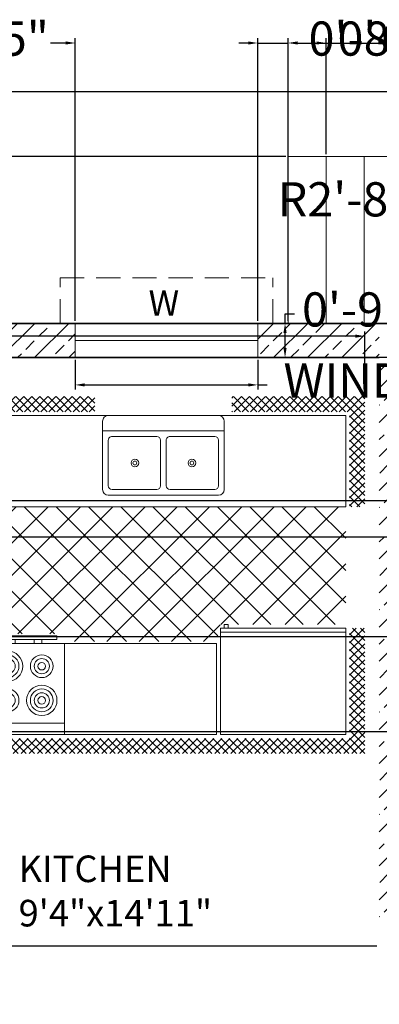
# Model space of a CAD drawing. Units: inches. Extents: x 9689 to 10369, y 10965 to 11626.
# Tile 6 of 11: x 9828 to 9923, y 11359 to 11619. Entities that reach past the tile are written whole.
import ezdxf

# ---------------------------------------------------------------- set-up
doc = ezdxf.new("R2010")
doc.units = ezdxf.units.IN
doc.linetypes.add('DASHED2', pattern=[9.525, 6.35, -3.175])
for name, color, linetype, lineweight in [('A-ANNO-DIMS', 2, 'Continuous', 18), ('A-ANNO-TEXT', 7, 'Continuous', 18), ('A-AREA-IDEN', 7, 'Continuous', 18), ('A-FLOR-FIXT', 8, 'Continuous', 18), ('A-FLOR-STRS', 7, 'Continuous', 18), ('A-GLAZ', 4, 'Continuous', 18), ('A-GLAZ-OVHD', 4, 'DASHED2', 13), ('A-WALL', 7, 'Continuous', 35), ('A-WALL-PATT', 252, 'Continuous', 13)]:
    doc.layers.add(name, color=color, linetype=linetype, lineweight=lineweight)
doc.styles.get("Standard").update_dxf_attribs({"font": 'arial.ttf'})
doc.dimstyles.new('ISO-25', dxfattribs={"dimtxt": 9, "dimasz": 2.5, "dimexe": 1.25, "dimexo": 0.625, "dimgap": 2, "dimtad": 0, "dimtih": 1, "dimtoh": 1, "dimdec": 1, "dimlunit": 4, "dimtxsty": 'Standard', "dimcen": 2.5, "dimadec": 0, "dimazin": 0, "dimtfac": 0.5, "dimtdec": 1, "dimtmove": 0, "dimatfit": 3, "dimfxl": 1, "dimarcsym": 0})

# ---------------------------------------------------------------- blocks, each defined once
blk = doc.blocks.new('Kitchen Layout - 7 x 8 ft')
for p, q in [((-5, 81.32), (2.68, 89)), ((-5, 83.44), (0.56, 89)), ((-5, 85.56), (-1.56, 89)), ((-5, 87.68), (-3.68, 89)), ((-1, 84.97), (-5, 88.97)), ((1.09, 85), (-2.91, 89)), ((3.21, 85), (-0.79, 89)), ((0.81, 85), (4.81, 89)), ((5.34, 85), (1.34, 89)), ((2.93, 85), (6.93, 89)), ((7.46, 85), (3.46, 89)), ((5.05, 85), (9.05, 89)), ((9.58, 85), (5.58, 89)), ((7.17, 85), (11.17, 89)), ((11.7, 85), (7.7, 89)), ((9.29, 85), (13.29, 89)), ((13.82, 85), (9.82, 89)), ((11.41, 85), (15.41, 89)), ((15.94, 85), (11.94, 89)), ((13.53, 85), (17.53, 89)), ((18.06, 85), (14.06, 89)), ((15.65, 85), (19.65, 89)), ((20.18, 85), (16.18, 89)), ((17.78, 85), (21.78, 89)), ((22.31, 85), (18.31, 89)), ((19.9, 85), (23.9, 89)), ((24.43, 85), (20.43, 89)), ((22.02, 85), (26.02, 89)), ((26.55, 85), (22.55, 89)), ((24.14, 85), (28.14, 89)), ((28.67, 85), (24.67, 89)), ((26.26, 85), (30.26, 89)), ((30.79, 85), (26.79, 89)), ((28.38, 85), (32.38, 89)), ((32.91, 85), (28.91, 89)), ((30.5, 85), (34.5, 89)), ((35.03, 85), (31.03, 89)), ((32.63, 85), (36.63, 89)), ((37.16, 85), (33.16, 89)), ((34.75, 85), (38.75, 89)), ((39.28, 85), (35.28, 89)), ((36.87, 85), (40.87, 89)), ((41.4, 85), (37.4, 89)), ((38.99, 85), (42.99, 89)), ((43.52, 85), (39.52, 89)), ((41.11, 85), (45.11, 89)), ((45.64, 85), (41.64, 89)), ((43.23, 85), (47.23, 89)), ((47.76, 85), (43.76, 89)), ((45.35, 85), (49.35, 89)), ((49.88, 85), (45.88, 89)), ((47.47, 85), (51.47, 89)), ((52, 85), (48, 89)), ((49.6, 85), (53.6, 89)), ((54.13, 85), (50.13, 89)), ((51.72, 85), (55.72, 89)), ((56.25, 85), (52.25, 89)), ((53.84, 85), (57.84, 89)), ((58.37, 85), (54.37, 89)), ((55.96, 85), (59.96, 89)), ((60.49, 85), (56.49, 89)), ((58.08, 85), (62.08, 89)), ((62.61, 85), (58.61, 89)), ((60.2, 85), (64.2, 89)), ((64.73, 85), (60.73, 89)), ((62.32, 85), (66.32, 89)), ((66.85, 85), (62.85, 89)), ((64.45, 85), (68.45, 89)), ((68.97, 85), (64.97, 89)), ((66.57, 85), (70.57, 89)), ((71.1, 85), (67.1, 89)), ((68.69, 85), (72.69, 89)), ((73.22, 85), (69.22, 89)), ((70.81, 85), (74.81, 89)), ((75.34, 85), (71.34, 89)), ((72.93, 85), (76.93, 89)), ((77.46, 85), (73.46, 89)), ((75.05, 85), (79.05, 89)), ((79.58, 85), (75.58, 89)), ((77.17, 85), (81.17, 89)), ((81.7, 85), (77.7, 89)), ((79.29, 85), (83.29, 89)), ((83.82, 85), (79.82, 89)), ((81.42, 85), (85.42, 89)), ((85.95, 85), (81.95, 89)), ((83.54, 85), (87.54, 89)), ((88.07, 85), (84.07, 89)), ((85.66, 85), (89.66, 89)), ((90.19, 85), (86.19, 89)), ((87.78, 85), (91.78, 89)), ((92.31, 85), (88.31, 89)), ((89.9, 85), (93.9, 89)), ((94.43, 85), (90.43, 89)), ((92.02, 85), (96.02, 89)), ((96.55, 85), (92.55, 89)), ((94.14, 85), (98.14, 89)), ((101, 82.67), (94.67, 89)), ((96.27, 85), (100.27, 89)), ((101, 84.79), (96.79, 89)), ((101, 86.92), (98.92, 89)), ((-1, 82.85), (-5, 86.85)), ((97, 83.61), (101, 87.61)), ((-1, 80.73), (-5, 84.73)), ((-5, 79.19), (-1, 83.19)), ((34, 84), (96, 84)), ((34, 60), (34, 84)), ((96, 84), (96, 60)), ((97, 81.49), (101, 85.49)), ((101, 80.55), (97, 84.55)), ((97, 79.37), (101, 83.37)), ((-1, 78.61), (-5, 82.61)), ((-5, 77.07), (-1, 81.07)), ((-1, 76.49), (-5, 80.49)), ((74, 81), (95, 81)), ((101, 78.43), (97, 82.43)), ((97, 77.25), (101, 81.25)), ((-5, 74.95), (-1, 78.95)), ((-1, 74.36), (-5, 78.36)), ((101, 76.31), (97, 80.31)), ((97, 75.13), (101, 79.13)), ((101, 74.19), (97, 78.19)), ((-5, 72.83), (-1, 76.83)), ((-1, 72.24), (-5, 76.24)), ((97, 73.01), (101, 77.01)), ((101, 72.07), (97, 76.07)), ((-5, 70.71), (-1, 74.71)), ((-1, 70.12), (-5, 74.12)), ((-5, 68.59), (-1, 72.59)), ((97, 70.89), (101, 74.89)), ((101, 69.95), (97, 73.95)), ((97, 68.76), (101, 72.76)), ((-1, 68), (-5, 72)), ((-5, 66.47), (-1, 70.47)), ((101, 67.82), (97, 71.82)), ((97, 66.64), (101, 70.64)), ((-1, 65.88), (-5, 69.88)), ((-5, 64.35), (-1, 68.35)), ((-1, 63.76), (-5, 67.76)), ((101, 65.7), (97, 69.7)), ((97, 64.52), (101, 68.52)), ((101, 63.58), (97, 67.58)), ((-5, 62.22), (-1, 66.22)), ((-1, 61.64), (-5, 65.64)), ((97, 62.4), (101, 66.4)), ((101, 61.46), (97, 65.46)), ((-5, 60.1), (-1, 64.1)), ((-1, 59.52), (-5, 63.52)), ((97, 60.28), (101, 64.28)), ((100.34, 60), (97, 63.34)), ((-5, 57.98), (-1, 61.98)), ((-1, 57.39), (-5, 61.39)), ((-4.86, 56), (-1, 59.86)), ((96, 60), (34, 60)), ((80, 60), (80, 59)), ((82, 59), (82, 60)), ((87, 59), (87, 60)), ((89, 60), (89, 59)), ((98.22, 60), (97, 61.22)), ((98.84, 60), (101, 62.16)), ((100.96, 60), (101, 60.04)), ((-1.73, 56), (-5, 59.27)), ((-3.85, 56), (-5, 57.15)), ((-2.74, 56), (-1, 57.74)), ((10.4, 24), (45.9, 59.5)), ((18.88, 24), (54.38, 59.5)), ((27.37, 24), (62.87, 59.5)), ((33.03, 55.11), (37.41, 59.5)), ((67.71, 24), (33.68, 58.04)), ((35.85, 24), (71.35, 59.5)), ((76.2, 24), (40.7, 59.5)), ((44.34, 24), (77.84, 57.5)), ((84.68, 24), (49.18, 59.5)), ((52.82, 24), (86.32, 57.5)), ((93.17, 24), (57.67, 59.5)), ((61.31, 24), (96, 58.69)), ((96, 29.65), (66.15, 59.5)), ((96, 38.14), (76.64, 57.5)), ((96, 46.63), (85.13, 57.5)), ((96, 55.11), (93.57, 57.54)), ((0, 57), (33, 57)), ((0, 30.57), (24.43, 55)), ((0, 39.06), (15.94, 55)), ((0, 47.54), (7.46, 55)), ((1.91, 24), (32.91, 55)), ((33.77, 24), (2.77, 55)), ((42.26, 24), (11.26, 55)), ((50.74, 24), (19.74, 55)), ((59.23, 24), (28.23, 55)), ((31, 55), (31, 56)), ((32, 55), (31, 55)), ((32, 56), (32, 55)), ((25.29, 24), (0, 49.29)), ((69.79, 24), (96, 50.21)), ((78.28, 24), (96, 41.72)), ((16.8, 24), (0, 40.8)), ((8.32, 24), (0, 32.32)), ((86.76, 24), (96, 33.24)), ((-5, 21.92), (-2.92, 24)), ((-5, 19.8), (-1, 23.8)), ((-1, 21.33), (-3.67, 24)), ((-1, 23.45), (-1.55, 24)), ((0, 24), (96, 24)), ((0, 0), (0, 24)), ((95.25, 24), (96, 24.75)), ((96, 24), (96, 0)), ((97, 22.1), (98.9, 24)), ((97, 19.97), (101, 23.97)), ((101, 21.16), (98.16, 24)), ((101, 23.28), (100.28, 24)), ((-1, 19.21), (-5, 23.21)), ((-5, 17.68), (-1, 21.68)), ((-1, 17.09), (-5, 21.09)), ((101, 19.03), (97, 23.03)), ((97, 17.85), (101, 21.85)), ((101, 16.91), (97, 20.91)), ((-5, 15.55), (-1, 19.55)), ((-1, 14.97), (-5, 18.97)), ((47.25, 6.5), (47.25, 18.5)), ((48.75, 18.5), (48.75, 6.5)), ((97, 15.73), (101, 19.73)), ((101, 14.79), (97, 18.79)), ((-5, 13.43), (-1, 17.43)), ((-1, 12.85), (-5, 16.85)), ((97, 13.61), (101, 17.61)), ((101, 12.67), (97, 16.67)), ((-5, 11.31), (-1, 15.31)), ((-1, 10.73), (-5, 14.73)), ((-5, 9.19), (-1, 13.19)), ((97, 11.49), (101, 15.49)), ((101, 10.55), (97, 14.55)), ((97, 9.37), (101, 13.37)), ((-1, 8.6), (-5, 12.6)), ((-5, 7.07), (-1, 11.07)), ((-1, 6.48), (-5, 10.48)), ((101, 8.43), (97, 12.43)), ((97, 7.25), (101, 11.25)), ((-5, 4.95), (-1, 8.95)), ((-1, 4.36), (-5, 8.36)), ((101, 6.31), (97, 10.31)), ((97, 5.12), (101, 9.12)), ((101, 4.18), (97, 8.18)), ((-5, 2.83), (-1, 6.83)), ((-1, 2.24), (-5, 6.24)), ((97, 3), (101, 7)), ((101, 2.06), (97, 6.06)), ((-5, 0.71), (-1, 4.71)), ((-1, 0.12), (-5, 4.12)), ((64, 4), (32, 4)), ((93.24, -5), (101, 2.76)), ((97, 0.88), (101, 4.88)), ((101, -0.06), (97, 3.94)), ((-5, -1.42), (-1, 2.58)), ((2, -5), (-5, 2)), ((-5, -3.54), (-1, 0.46)), ((96, 0), (0, 0)), ((95.36, -5), (101, 0.64)), ((101, -2.18), (97, 1.82)), ((-0.12, -5), (-5, -0.12)), ((-2.25, -5), (-5, -2.25)), ((-4.34, -5), (-0.34, -1)), ((-2.22, -5), (1.78, -1)), ((-0.1, -5), (3.9, -1)), ((4.12, -5), (0.12, -1)), ((2.02, -5), (6.02, -1)), ((6.24, -5), (2.24, -1)), ((4.14, -5), (8.14, -1)), ((8.36, -5), (4.36, -1)), ((6.27, -5), (10.27, -1)), ((10.48, -5), (6.48, -1)), ((8.39, -5), (12.39, -1)), ((12.6, -5), (8.6, -1)), ((10.51, -5), (14.51, -1)), ((14.73, -5), (10.73, -1)), ((12.63, -5), (16.63, -1)), ((16.85, -5), (12.85, -1)), ((14.75, -5), (18.75, -1)), ((18.97, -5), (14.97, -1)), ((16.87, -5), (20.87, -1)), ((21.09, -5), (17.09, -1)), ((18.99, -5), (22.99, -1)), ((23.21, -5), (19.21, -1)), ((21.11, -5), (25.11, -1)), ((25.33, -5), (21.33, -1)), ((23.24, -5), (27.24, -1)), ((27.45, -5), (23.45, -1)), ((25.36, -5), (29.36, -1)), ((29.57, -5), (25.57, -1)), ((27.48, -5), (30, -2.48)), ((30, -3.3), (27.7, -1)), ((30, -1.18), (29.82, -1)), ((66, -2.54), (67.54, -1)), ((66, -4.66), (69.66, -1)), ((69.88, -5), (66, -1.12)), ((67.78, -5), (71.78, -1)), ((72, -5), (68, -1)), ((69.9, -5), (73.9, -1)), ((74.12, -5), (70.12, -1)), ((72.03, -5), (76.03, -1)), ((76.24, -5), (72.24, -1)), ((74.15, -5), (78.15, -1)), ((78.36, -5), (74.36, -1)), ((76.27, -5), (80.27, -1)), ((80.49, -5), (76.49, -1)), ((78.39, -5), (82.39, -1)), ((82.61, -5), (78.61, -1)), ((80.51, -5), (84.51, -1)), ((84.73, -5), (80.73, -1)), ((82.63, -5), (86.63, -1)), ((86.85, -5), (82.85, -1)), ((84.75, -5), (88.75, -1)), ((88.97, -5), (84.97, -1)), ((86.88, -5), (90.88, -1)), ((91.09, -5), (87.09, -1)), ((89, -5), (93, -1)), ((93.21, -5), (89.21, -1)), ((91.12, -5), (95.12, -1)), ((95.34, -5), (91.34, -1)), ((97.46, -5), (93.46, -1)), ((99.58, -5), (95.58, -1)), ((101, -4.3), (97, -0.3)), ((97.48, -5), (101, -1.48)), ((-4.37, -5), (-5, -4.37)), ((29.6, -5), (30, -4.6)), ((67.76, -5), (66, -3.24)), ((99.6, -5), (101, -3.6))]:
    blk.add_line(p, q)
for points in [[(0, 56), (0, 84), (33, 84), (33, 56)], [(74, 60), (74, 84), (95, 84), (95, 60)], [(76, 58), (76, 59), (93, 59), (93, 58)]]:
    blk.add_lwpolyline(points, close=True)
for points in [[(33.5, 21), (62.5, 21)], [(32, 1.5), (32, 19.5)], [(33.5, 6.5), (33.5, 18.5)], [(34.5, 19.5), (46.25, 19.5)], [(49.75, 19.5), (61.5, 19.5)], [(62.5, 18.5), (62.5, 6.5)], [(64, 19.5), (64, 1.5)], [(46.25, 5.5), (34.5, 5.5)], [(61.5, 5.5), (49.75, 5.5)], [(62.5, 0), (33.5, 0)]]:
    blk.add_lwpolyline(points)
for centre, radius in [((80, 75), 4), ((80, 75), 3), ((89, 75), 3), ((80, 75), 2), ((80, 75), 1), ((89, 75), 2), ((89, 75), 1), ((89, 66), 4), ((80, 66), 3), ((80, 66), 2), ((89, 66), 3), ((89, 66), 2), ((80, 66), 1), ((89, 66), 1), ((40.5, 12.5), 1), ((40.5, 12.5), 0.5), ((55.5, 12.5), 1), ((55.5, 12.5), 0.5)]:
    blk.add_circle(centre, radius)
for centre, radius, start, end in [((33.5, 19.5), 1.5, 90, 180), ((62.5, 19.5), 1.5, 0, 90), ((34.5, 18.5), 1, 90, 180), ((46.25, 18.5), 1, 0, 90), ((49.75, 18.5), 1, 90, 180), ((61.5, 18.5), 1, 0, 90), ((34.5, 6.5), 1, 180, 270), ((46.25, 6.5), 1, 270, 0), ((49.75, 6.5), 1, 180, 270), ((61.5, 6.5), 1, 270, 0), ((33.5, 1.5), 1.5, 180, 270), ((62.5, 1.5), 1.5, 270, 0)]:
    blk.add_arc(centre, radius, start, end)
blk = doc.blocks.new('*D21')
at = {"layer": 'A-ANNO-DIMS', "color": 0, "lineweight": -2, "transparency": 16777216}
for p, q in [((9802.06, 11539.26), (9802.06, 11600.92)), ((10244.06, 11539.26), (10244.06, 11600.92)), ((9804.56, 11599.67), (10002.11, 11599.67)), ((10241.56, 11599.67), (10044.01, 11599.67))]:
    blk.add_line(p, q, dxfattribs=at)
at = {"layer": 'A-ANNO-DIMS', "color": 0, "transparency": 16777216}
for points in [[(9804.56, 11600.08), (9804.56, 11599.25), (9802.06, 11599.67)], [(10241.56, 11600.08), (10241.56, 11599.25), (10244.06, 11599.67)]]:
    blk.add_solid(points, dxfattribs=at)
at = {"layer": 'Defpoints', "color": 0, "transparency": 16777216}
for p in [(10244.06, 11599.67), (9802.06, 11538.63), (10244.06, 11538.63)]:
    blk.add_point(p, dxfattribs=at)
at = {"layer": 'A-ANNO-DIMS', "color": 0, "transparency": 16777216, "insert": (10023.06, 11599.67), "char_height": 9, "attachment_point": 5}
blk.add_mtext('36\'-10"', dxfattribs=at)
blk = doc.blocks.new('WINDOW-HOOD-56')
for p, q in [((0, 0), (0, 12)), ((0, 12), (56, 12)), ((56, 0), (56, 12))]:
    blk.add_line(p, q)
blk = doc.blocks.new('WINDOW-48')
for p, q in [((0, 0), (0, 9)), ((48, 0), (48, 9)), ((0, 4.5), (48, 4.5))]:
    blk.add_line(p, q)
blk = doc.blocks.new('*D42')
at = {"layer": 'A-ANNO-DIMS', "color": 0, "lineweight": -2, "transparency": 16777216}
for p, q in [((9843.06, 11529.01), (9843.06, 11521.18)), ((9891.06, 11529.01), (9891.06, 11521.18)), ((9845.56, 11522.43), (9888.56, 11522.43)), ((9891.06, 11522.43), (9893.56, 11522.43))]:
    blk.add_line(p, q, dxfattribs=at)
at = {"layer": 'A-ANNO-DIMS', "color": 0, "transparency": 16777216}
for points in [[(9845.56, 11522.85), (9845.56, 11522.01), (9843.06, 11522.43)], [(9888.56, 11522.85), (9888.56, 11522.01), (9891.06, 11522.43)]]:
    blk.add_solid(points, dxfattribs=at)
at = {"layer": 'Defpoints', "color": 0, "transparency": 16777216}
for p in [(9843.06, 11529.63), (9891.06, 11529.63), (9891.06, 11522.43)]:
    blk.add_point(p, dxfattribs=at)
at = {"layer": 'A-ANNO-DIMS', "color": 0, "transparency": 16777216, "insert": (9952.5, 11522.43), "char_height": 9, "attachment_point": 5}
blk.add_mtext('WINDOW 4\'-0" TYP.', dxfattribs=at)
blk = doc.blocks.new('*D43')
at = {"layer": 'A-ANNO-DIMS', "color": 0, "lineweight": -2, "transparency": 16777216}
for p, q in [((9898.26, 11538.63), (9898.26, 11541.13)), ((9898.26, 11541.13), (9900.76, 11541.13)), ((9891.68, 11538.63), (9899.51, 11538.63)), ((9898.26, 11532.13), (9898.26, 11536.13)), ((9891.68, 11529.63), (9899.51, 11529.63))]:
    blk.add_line(p, q, dxfattribs=at)
at = {"layer": 'A-ANNO-DIMS', "color": 0, "transparency": 16777216}
for points in [[(9897.84, 11536.13), (9898.67, 11536.13), (9898.26, 11538.63)], [(9897.84, 11532.13), (9898.67, 11532.13), (9898.26, 11529.63)]]:
    blk.add_solid(points, dxfattribs=at)
at = {"layer": 'Defpoints', "color": 0, "transparency": 16777216}
for p in [(9891.06, 11538.63), (9898.26, 11538.63), (9891.06, 11529.63)]:
    blk.add_point(p, dxfattribs=at)
at = {"layer": 'A-ANNO-DIMS', "color": 0, "transparency": 16777216, "insert": (9930.19, 11541.13), "char_height": 9, "attachment_point": 5}
blk.add_mtext('0\'-9" TYP.', dxfattribs=at)
blk = doc.blocks.new('*D50')
at = {"layer": 'A-ANNO-DIMS', "color": 0, "lineweight": -2, "transparency": 16777216}
for p, q in [((9813.25, 11519.99), (9813.25, 11536.52)), ((9919.25, 11519.99), (9919.25, 11536.52)), ((9813.25, 11535.27), (9810.75, 11535.27)), ((9916.75, 11535.27), (9815.75, 11535.27))]:
    blk.add_line(p, q, dxfattribs=at)
at = {"layer": 'A-ANNO-DIMS', "color": 0, "transparency": 16777216}
for points in [[(9815.75, 11535.69), (9815.75, 11534.85), (9813.25, 11535.27)], [(9916.75, 11535.69), (9916.75, 11534.85), (9919.25, 11535.27)]]:
    blk.add_solid(points, dxfattribs=at)
at = {"layer": 'Defpoints', "color": 0, "transparency": 16777216}
for p in [(9813.25, 11535.27), (9813.25, 11519.37), (9919.25, 11519.37)]:
    blk.add_point(p, dxfattribs=at)
at = {"layer": 'A-ANNO-DIMS', "color": 0, "transparency": 16777216, "insert": (9747.74, 11535.27), "char_height": 9, "attachment_point": 5}
blk.add_mtext('KITCHEN UNIT 8\'-10"', dxfattribs=at)
blk = doc.blocks.new('*D80')
at = {"layer": 'A-ANNO-DIMS', "color": 0, "lineweight": -2, "transparency": 16777216}
for p, q in [((9979.43, 11529.63), (9758.91, 11529.63)), ((9760.16, 11527.13), (9760.16, 11512.66)), ((9760.16, 11484.88), (9760.16, 11499.35)), ((9979.43, 11482.38), (9758.91, 11482.38))]:
    blk.add_line(p, q, dxfattribs=at)
at = {"layer": 'A-ANNO-DIMS', "color": 0, "transparency": 16777216}
for points in [[(9759.74, 11527.13), (9760.57, 11527.13), (9760.16, 11529.63)], [(9759.74, 11484.88), (9760.57, 11484.88), (9760.16, 11482.38)]]:
    blk.add_solid(points, dxfattribs=at)
at = {"layer": 'Defpoints', "color": 0, "transparency": 16777216}
for p in [(9760.16, 11529.63), (9980.06, 11529.63), (9980.06, 11482.38)]:
    blk.add_point(p, dxfattribs=at)
at = {"layer": 'A-ANNO-DIMS', "color": 0, "transparency": 16777216, "insert": (9760.16, 11506.01), "char_height": 9, "attachment_point": 5}
blk.add_mtext('3\'-11 1/2"', dxfattribs=at)
blk = doc.blocks.new('*D82')
at = {"layer": 'A-ANNO-DIMS', "color": 0, "lineweight": -2, "transparency": 16777216}
for p, q in [((9898.43, 11582.55), (9758.91, 11582.55)), ((9760.16, 11580.05), (9760.16, 11567.19)), ((9760.16, 11541.13), (9760.16, 11553.99)), ((9898.43, 11538.63), (9758.91, 11538.63))]:
    blk.add_line(p, q, dxfattribs=at)
at = {"layer": 'A-ANNO-DIMS', "color": 0, "transparency": 16777216}
for points in [[(9759.74, 11580.05), (9760.57, 11580.05), (9760.16, 11582.55)], [(9759.74, 11541.13), (9760.57, 11541.13), (9760.16, 11538.63)]]:
    blk.add_solid(points, dxfattribs=at)
at = {"layer": 'Defpoints', "color": 0, "transparency": 16777216}
for p in [(9760.16, 11582.55), (9899.06, 11582.55), (9899.06, 11538.63)]:
    blk.add_point(p, dxfattribs=at)
at = {"layer": 'A-ANNO-DIMS', "color": 0, "transparency": 16777216, "insert": (9760.16, 11560.59), "char_height": 9, "attachment_point": 5}
blk.add_mtext('3\'-8"', dxfattribs=at)
blk = doc.blocks.new('*D83')
at = {"layer": 'A-ANNO-DIMS', "color": 0, "lineweight": -2, "transparency": 16777216}
for p, q in [((9899.06, 11583.18), (9899.06, 11613.7)), ((9901.56, 11612.45), (9923.07, 11612.45)), ((9972.56, 11612.45), (9951.04, 11612.45)), ((9975.06, 11583.18), (9975.06, 11613.7))]:
    blk.add_line(p, q, dxfattribs=at)
at = {"layer": 'A-ANNO-DIMS', "color": 0, "transparency": 16777216}
for points in [[(9901.56, 11612.87), (9901.56, 11612.04), (9899.06, 11612.45)], [(9972.56, 11612.87), (9972.56, 11612.04), (9975.06, 11612.45)]]:
    blk.add_solid(points, dxfattribs=at)
at = {"layer": 'Defpoints', "color": 0, "transparency": 16777216}
for p in [(9975.06, 11612.45), (9899.06, 11582.55), (9975.06, 11582.55)]:
    blk.add_point(p, dxfattribs=at)
at = {"layer": 'A-ANNO-DIMS', "color": 0, "transparency": 16777216, "insert": (9937.06, 11612.45), "char_height": 9, "attachment_point": 5}
blk.add_mtext('6\'-4"', dxfattribs=at)
blk = doc.blocks.new('*D86')
at = {"layer": 'A-ANNO-DIMS', "color": 0, "lineweight": -2, "transparency": 16777216}
for p, q in [((9802.06, 11539.26), (9802.06, 11613.7)), ((9804.56, 11612.45), (9808.6, 11612.45)), ((9840.56, 11612.45), (9836.52, 11612.45)), ((9843.06, 11539.26), (9843.06, 11613.7))]:
    blk.add_line(p, q, dxfattribs=at)
at = {"layer": 'A-ANNO-DIMS', "color": 0, "transparency": 16777216}
for points in [[(9804.56, 11612.87), (9804.56, 11612.04), (9802.06, 11612.45)], [(9840.56, 11612.87), (9840.56, 11612.04), (9843.06, 11612.45)]]:
    blk.add_solid(points, dxfattribs=at)
at = {"layer": 'Defpoints', "color": 0, "transparency": 16777216}
for p in [(9843.06, 11612.45), (9802.06, 11538.63), (9843.06, 11538.63)]:
    blk.add_point(p, dxfattribs=at)
at = {"layer": 'A-ANNO-DIMS', "color": 0, "transparency": 16777216, "insert": (9822.56, 11612.45), "char_height": 9, "attachment_point": 5}
blk.add_mtext('3\'-5"', dxfattribs=at)
blk = doc.blocks.new('*D99')
at = {"layer": 'A-ANNO-DIMS', "color": 0, "lineweight": -2, "transparency": 16777216}
for p, q in [((9922.43, 11374.63), (9758.91, 11374.63)), ((9760.16, 11372.13), (9760.16, 11357.23)), ((9760.16, 11329.13), (9760.16, 11344.03)), ((9801.43, 11326.63), (9758.91, 11326.63))]:
    blk.add_line(p, q, dxfattribs=at)
at = {"layer": 'A-ANNO-DIMS', "color": 0, "transparency": 16777216}
for points in [[(9759.74, 11372.13), (9760.57, 11372.13), (9760.16, 11374.63)], [(9759.74, 11329.13), (9760.57, 11329.13), (9760.16, 11326.63)]]:
    blk.add_solid(points, dxfattribs=at)
at = {"layer": 'Defpoints', "color": 0, "transparency": 16777216}
for p in [(9923.06, 11374.63), (9760.16, 11326.63), (9802.06, 11326.63)]:
    blk.add_point(p, dxfattribs=at)
at = {"layer": 'A-ANNO-DIMS', "color": 0, "transparency": 16777216, "insert": (9760.16, 11350.63), "char_height": 9, "attachment_point": 5}
blk.add_mtext('4\'-0"', dxfattribs=at)
blk = doc.blocks.new('*D101')
at = {"layer": 'A-ANNO-DIMS', "color": 0, "lineweight": -2, "transparency": 16777216}
for p, q in [((9888.56, 11612.45), (9886.06, 11612.45)), ((9891.06, 11539.26), (9891.06, 11613.7)), ((9891.06, 11612.45), (9899.06, 11612.45)), ((9899.06, 11539.26), (9899.06, 11613.7)), ((9901.56, 11612.45), (9904.06, 11612.45))]:
    blk.add_line(p, q, dxfattribs=at)
at = {"layer": 'A-ANNO-DIMS', "color": 0, "transparency": 16777216}
for points in [[(9888.56, 11612.87), (9888.56, 11612.04), (9891.06, 11612.45)], [(9901.56, 11612.87), (9901.56, 11612.04), (9899.06, 11612.45)]]:
    blk.add_solid(points, dxfattribs=at)
at = {"layer": 'Defpoints', "color": 0, "transparency": 16777216}
for p in [(9899.06, 11612.45), (9891.06, 11538.63), (9899.06, 11538.63)]:
    blk.add_point(p, dxfattribs=at)
at = {"layer": 'A-ANNO-DIMS', "color": 0, "transparency": 16777216, "insert": (9918.02, 11612.45), "char_height": 9, "attachment_point": 5}
blk.add_mtext('0\'-8"', dxfattribs=at)
blk = doc.blocks.new('*D108')
at = {"layer": 'A-ANNO-DIMS', "color": 0, "lineweight": -2, "transparency": 16777216}
for p, q in [((9922.43, 11529.63), (9758.91, 11529.63)), ((9760.16, 11527.13), (9760.16, 11458.65)), ((9760.16, 11377.13), (9760.16, 11445.61)), ((9922.43, 11374.63), (9758.91, 11374.63))]:
    blk.add_line(p, q, dxfattribs=at)
at = {"layer": 'A-ANNO-DIMS', "color": 0, "transparency": 16777216}
for points in [[(9759.74, 11527.13), (9760.57, 11527.13), (9760.16, 11529.63)], [(9759.74, 11377.13), (9760.57, 11377.13), (9760.16, 11374.63)]]:
    blk.add_solid(points, dxfattribs=at)
at = {"layer": 'Defpoints', "color": 0, "transparency": 16777216}
for p in [(9760.16, 11529.63), (9923.06, 11529.63), (9923.06, 11374.63)]:
    blk.add_point(p, dxfattribs=at)
at = {"layer": 'A-ANNO-DIMS', "color": 0, "transparency": 16777216, "insert": (9760.16, 11452.13), "char_height": 9, "attachment_point": 5}
blk.add_mtext('12\'-11"', dxfattribs=at)
blk = doc.blocks.new('*D110')
at = {"layer": 'A-ANNO-DIMS', "color": 0, "lineweight": -2, "transparency": 16777216}
for p, q in [((10021.43, 11456.13), (9758.91, 11456.13)), ((9760.16, 11453.63), (9760.16, 11450.15)), ((9760.16, 11433.63), (9760.16, 11437.11)), ((10021.43, 11431.13), (9758.91, 11431.13))]:
    blk.add_line(p, q, dxfattribs=at)
at = {"layer": 'A-ANNO-DIMS', "color": 0, "transparency": 16777216}
for points in [[(9759.74, 11453.63), (9760.57, 11453.63), (9760.16, 11456.13)], [(9759.74, 11433.63), (9760.57, 11433.63), (9760.16, 11431.13)]]:
    blk.add_solid(points, dxfattribs=at)
at = {"layer": 'Defpoints', "color": 0, "transparency": 16777216}
for p in [(9760.16, 11456.13), (10022.06, 11456.13), (10022.06, 11431.13)]:
    blk.add_point(p, dxfattribs=at)
at = {"layer": 'A-ANNO-DIMS', "color": 0, "transparency": 16777216, "insert": (9760.16, 11443.63), "char_height": 9, "attachment_point": 5}
blk.add_mtext('2\'-1"', dxfattribs=at)
blk = doc.blocks.new('*D111')
at = {"layer": 'A-ANNO-DIMS', "color": 0, "lineweight": -2, "transparency": 16777216}
for p, q in [((9899.06, 11583.18), (9899.06, 11613.7)), ((9901.56, 11612.45), (9906.56, 11612.45)), ((9909.06, 11583.18), (9909.06, 11613.7)), ((9909.06, 11612.45), (9911.56, 11612.45))]:
    blk.add_line(p, q, dxfattribs=at)
at = {"layer": 'A-ANNO-DIMS', "color": 0, "transparency": 16777216}
for points in [[(9901.56, 11612.87), (9901.56, 11612.04), (9899.06, 11612.45)], [(9906.56, 11612.87), (9906.56, 11612.04), (9909.06, 11612.45)]]:
    blk.add_solid(points, dxfattribs=at)
at = {"layer": 'Defpoints', "color": 0, "transparency": 16777216}
for p in [(9909.06, 11612.45), (9899.06, 11582.55), (9909.06, 11582.55)]:
    blk.add_point(p, dxfattribs=at)
at = {"layer": 'A-ANNO-DIMS', "color": 0, "transparency": 16777216, "insert": (9929.02, 11612.45), "char_height": 9, "attachment_point": 5}
blk.add_mtext('0\'-10"', dxfattribs=at)
blk = doc.blocks.new('*D118')
at = {"layer": 'A-ANNO-DIMS', "color": 0, "lineweight": -2, "transparency": 16777216}
for p, q in [((9980.91, 11491.91), (9758.91, 11491.91)), ((9760.16, 11489.41), (9760.16, 11484.88)), ((9979.43, 11482.38), (9758.91, 11482.38)), ((9760.16, 11482.38), (9760.16, 11479.88)), ((9760.16, 11479.88), (9757.66, 11479.88))]:
    blk.add_line(p, q, dxfattribs=at)
at = {"layer": 'A-ANNO-DIMS', "color": 0, "transparency": 16777216}
for points in [[(9759.74, 11489.41), (9760.57, 11489.41), (9760.16, 11491.91)], [(9759.74, 11484.88), (9760.57, 11484.88), (9760.16, 11482.38)]]:
    blk.add_solid(points, dxfattribs=at)
at = {"layer": 'Defpoints', "color": 0, "transparency": 16777216}
for p in [(9981.53, 11491.91), (9760.16, 11482.38), (9980.06, 11482.38)]:
    blk.add_point(p, dxfattribs=at)
at = {"layer": 'A-ANNO-DIMS', "color": 0, "transparency": 16777216, "insert": (9733.21, 11479.88), "char_height": 9, "attachment_point": 5}
blk.add_mtext('0\'-9 1/2"', dxfattribs=at)
blk = doc.blocks.new('*D120')
at = {"layer": 'A-ANNO-DIMS', "color": 0, "lineweight": -2, "transparency": 16777216}
for p, q in [((9932.06, 11570.13), (9934.56, 11570.13)), ((9934.56, 11570.13), (9946.29, 11558.4)), ((9970.56, 11534.13), (9948.06, 11556.63))]:
    blk.add_line(p, q, dxfattribs=at)
at = {"layer": 'A-ANNO-DIMS', "color": 0, "transparency": 16777216}
blk.add_solid([(9946.58, 11558.69), (9945.99, 11558.1), (9948.06, 11556.63)], dxfattribs=at)
at = {"layer": 'Defpoints', "color": 0, "transparency": 16777216}
for p in [(9948.06, 11556.63), (9970.56, 11534.13)]:
    blk.add_point(p, dxfattribs=at)
at = {"layer": 'A-ANNO-DIMS', "color": 0, "transparency": 16777216, "insert": (9913.79, 11570.13), "char_height": 9, "attachment_point": 5}
blk.add_mtext('R2\'-8"', dxfattribs=at)

msp = doc.modelspace()

# ---------------------------------------------------------------- hatches: boundary and pattern name
at = {"layer": 'A-WALL-PATT'}
h = msp.add_hatch(dxfattribs=at)
h.set_pattern_fill('ANSI33', color=256)
h.paths.add_polyline_path([(9843.06, 11538.63), (9811.06, 11538.63), (9811.06, 11529.63), (9843.06, 11529.63)])
h.paths.add_polyline_path([(9923.06, 11538.63), (9891.06, 11538.63), (9891.06, 11529.63), (9923.06, 11529.63)])
h.paths.add_polyline_path([(9929.06, 11527.63), (9923.06, 11527.63), (9923.06, 11380.63), (9929.06, 11380.63)])
h.paths.add_polyline_path([(9939.06, 11538.63), (9929.06, 11538.63), (9929.06, 11529.63), (9939.06, 11529.63, -0.071068)])
h.paths.add_polyline_path([(10035.06, 11538.63), (10013.06, 11538.63), (10013.06, 11529.63), (10022.06, 11529.63), (10022.06, 11507.38), (10022.06, 11502.38), (10022.06, 11482.38), (10022.06, 11478.38), (10022.06, 11456.13, -0.038405), (10026.06, 11456.13), (10026.06, 11502.38), (10026.06, 11529.63), (10035.06, 11529.63)])
h.paths.add_polyline_path([(10068.06, 11538.63), (10059.06, 11538.63), (10059.06, 11529.63), (10068.06, 11529.63)])
h.paths.add_polyline_path([(10074.06, 11527.63), (10068.06, 11527.63), (10068.06, 11431.13), (10026.06, 11431.13), (10022.06, 11431.13), (9980.06, 11431.13), (9976.06, 11431.13), (9976.06, 11425.13), (10068.06, 11425.13), (10068.06, 11380.63), (10074.06, 11380.63)])
h.paths.add_polyline_path([(10124.56, 11538.63), (10074.06, 11538.63), (10074.06, 11529.63), (10124.56, 11529.63)])
h.paths.add_polyline_path([(9980.06, 11507.38), (9980.06, 11529.63), (9989.06, 11529.63), (9989.06, 11538.63), (9976.06, 11538.63), (9976.06, 11529.63), (9976.06, 11503.38), (9976.06, 11483.38), (9976.06, 11478.38), (9980.06, 11478.38), (9997.06, 11478.38, -0.038405), (9997.06, 11482.38), (9980.06, 11482.38)])
h.paths.add_polyline_path([(10235.06, 11538.63), (10184.56, 11538.63), (10184.56, 11529.63), (10235.06, 11529.63)])
h.paths.add_polyline_path([(10244.06, 11527.63), (10235.06, 11527.63), (10235.06, 11485.13), (10244.06, 11485.13)])
h.paths.add_polyline_path([(10244.06, 11425.13), (10235.06, 11425.13), (10235.06, 11380.63), (10244.06, 11380.63)])
h.paths.add_polyline_path([(10233.06, 11380.63), (10120.06, 11380.63, -0.038405), (10120.06, 11374.63), (10133.04, 11374.63), (10133.04, 11326.63), (10120.06, 11326.63, -0.038405), (10120.06, 11320.63), (10149.19, 11320.63), (10149.19, 11326.63), (10136.04, 11326.63), (10136.04, 11374.63), (10233.06, 11374.63)])
h.paths.add_polyline_path([(10084.06, 11380.63), (10076.06, 11380.63), (10076.06, 11374.63), (10084.06, 11374.63)])
h.paths.add_polyline_path([(10244.06, 11374.63), (10235.06, 11374.63), (10235.06, 11362.63), (10244.06, 11362.63)])
h.paths.add_polyline_path([(10244.06, 11338.63), (10235.06, 11338.63), (10235.06, 11326.63), (10244.06, 11326.63)])
h.paths.add_polyline_path([(10233.06, 11326.63), (10173.19, 11326.63, -0.055385), (10173.19, 11320.63), (10233.06, 11320.63)], flags=0)
h.paths.add_polyline_path([(10244.06, 11320.63), (10235.06, 11320.63), (10235.06, 11273.63), (10244.06, 11273.63)])
h = msp.add_hatch(dxfattribs=at)
h.set_pattern_fill('ANSI36', color=256)
h.paths.add_polyline_path([(10233.06, 11326.63), (10173.19, 11326.63, -0.055385), (10173.19, 11320.63), (10233.06, 11320.63)])
h.paths.add_polyline_path([(10244.06, 11213.63), (10235.06, 11213.63), (10235.06, 11166.63), (10244.06, 11166.63)])
h.paths.add_polyline_path([(10233.06, 11166.63), (10184.56, 11166.63), (10184.56, 11157.63), (10233.06, 11157.63)])
h.paths.add_polyline_path([(10124.56, 11166.63), (10074.06, 11166.63), (10074.06, 11157.63), (10124.56, 11157.63)])
h.paths.add_polyline_path([(10074.06, 11318.63), (10068.06, 11318.63), (10068.06, 11168.63), (10074.06, 11168.63)])
h.paths.add_polyline_path([(10068.06, 11166.63), (10011.06, 11166.63), (10011.06, 11157.63), (10068.06, 11157.63)])
h.paths.add_polyline_path([(10011.06, 11318.63), (10005.06, 11318.63), (10005.06, 11168.63), (10011.06, 11168.63)])
h.paths.add_polyline_path([(10005.06, 11166.63), (9985.06, 11166.63), (9985.06, 11157.63), (10005.06, 11157.63)])
h.paths.add_polyline_path([(9937.06, 11166.63), (9898.06, 11166.63), (9898.06, 11157.63), (9937.06, 11157.63, -0.042779)])
h.paths.add_polyline_path([(9850.06, 11166.63), (9813.06, 11166.63), (9813.06, 11157.63), (9850.06, 11157.63)])
h.paths.add_polyline_path([(9811.06, 11213.63), (9802.06, 11213.63), (9802.06, 11166.63), (9811.06, 11166.63)])
h.paths.add_polyline_path([(9811.06, 11320.63), (9802.06, 11320.63), (9802.06, 11273.63), (9811.06, 11273.63)])
h.paths.add_polyline_path([(9811.06, 11439.11), (9802.06, 11439.11), (9802.06, 11326.63), (9811.06, 11326.63)])
h.paths.add_polyline_path([(9957.06, 11326.63), (9813.06, 11326.63), (9813.06, 11320.63), (9957.06, 11320.63)])
h.paths.add_polyline_path([(9811.06, 11527.63), (9802.06, 11527.63), (9802.06, 11499.11), (9811.06, 11499.11)])

# ---------------------------------------------------------------- linework, layer by layer
at = {"layer": 'A-FLOR-STRS'}
for p, q in [((9899.06, 11538.63), (9899.06, 11582.55)), ((9899.06, 11582.55), (9929.06, 11582.55)), ((9909.06, 11538.63), (9909.06, 11582.55)), ((9919.06, 11538.63), (9919.06, 11582.55))]:
    msp.add_line(p, q, dxfattribs=at)
at = {"layer": 'A-WALL'}
for p, q in [((9802.06, 11538.63), (9939.06, 11538.63)), ((9811.06, 11529.63), (9923.06, 11529.63))]:
    msp.add_line(p, q, dxfattribs=at)

# ---------------------------------------------------------------- block references
at = {"layer": 'A-FLOR-FIXT', "rotation": 180}
msp.add_blockref('Kitchen Layout - 7 x 8 ft', (9914.25, 11514.37), dxfattribs=at)
at = {"layer": 'A-GLAZ'}
msp.add_blockref('WINDOW-48', (9843.06, 11529.63), dxfattribs=at)
at = {"layer": 'A-GLAZ-OVHD'}
msp.add_blockref('WINDOW-HOOD-56', (9839.06, 11538.63), dxfattribs=at)

# ---------------------------------------------------------------- texts
at = {"layer": 'A-ANNO-TEXT', "insert": (9862.34, 11547.36), "char_height": 6.729, "attachment_point": 1}
msp.add_mtext_dynamic_manual_height_columns('{\\fArial|b1|i0|c0|p34;W}', width=31.3623, gutter_width=33.65, heights=[0], dxfattribs=at)
at = {"layer": 'A-AREA-IDEN', "insert": (9828.15, 11398.52), "char_height": 7, "attachment_point": 1}
msp.add_mtext_dynamic_manual_height_columns('{\\fArial|b1|i0|c0|p34;KITCHEN\\P9\'4"x14\'11"}', width=85.4722, gutter_width=12.5, heights=[0], dxfattribs=at)

# ---------------------------------------------------------------- dimensions: what is measured, and where the dimension line sits
at = {"layer": 'A-ANNO-DIMS'}
for base, p1, p2, override, picture, middle in [((9843.06, 11612.45), (9802.06, 11538.63), (9843.06, 11538.63), {"dimdec": 1, "dimlfac": 1, "dimrnd": 0, "dimzin": 1, "dimdsep": 46, "dimlunit": 4, "dimfrac": 2}, '*D86', (9822.56, 11612.45)), ((9899.06, 11612.45), (9891.06, 11538.63), (9899.06, 11538.63), {"dimdec": 1, "dimlfac": 1, "dimrnd": 0, "dimzin": 1, "dimdsep": 46, "dimlunit": 4, "dimfrac": 2}, '*D101', (9918.02, 11612.45)), ((9975.06, 11612.45), (9899.06, 11582.55), (9975.06, 11582.55), {"dimdec": 1, "dimlfac": 1, "dimrnd": 0, "dimzin": 1, "dimdsep": 46, "dimlunit": 4, "dimfrac": 2}, '*D83', (9937.06, 11612.45)), ((9909.06, 11612.45), (9899.06, 11582.55), (9909.06, 11582.55), {"dimdec": 1, "dimlfac": 1, "dimrnd": 0, "dimzin": 1, "dimdsep": 46, "dimlunit": 4, "dimfrac": 2}, '*D111', (9929.02, 11612.45)), ((10244.06, 11599.67), (9802.06, 11538.63), (10244.06, 11538.63), {"dimclrd": 0, "dimclre": 0, "dimclrt": 0}, '*D21', (10023.06, 11599.67))]:
    dim = msp.add_linear_dim(base=base, p1=p1, p2=p2, dimstyle='ISO-25', override=override, dxfattribs=at)
    dim.commit()
    dim.dimension.update_dxf_attribs({"geometry": picture, "text_midpoint": middle})
for base, p1, p2, picture, middle in [((9760.16, 11582.55), (9899.06, 11538.63), (9899.06, 11582.55), '*D82', (9760.16, 11560.59)), ((9760.15676, 11529.630116), (9980.05676, 11482.380116), (9980.05676, 11529.630116), '*D80', (9760.15676, 11506.005116)), ((9760.16, 11529.63), (9923.06, 11374.63), (9923.06, 11529.63), '*D108', (9760.16, 11452.13)), ((9760.16, 11482.38), (9981.53, 11491.91), (9980.06, 11482.38), '*D118', (9733.21, 11479.88)), ((9760.16, 11456.13), (10022.06, 11431.13), (10022.06, 11456.13), '*D110', (9760.16, 11443.63)), ((9760.16, 11326.63), (9923.06, 11374.63), (9802.06, 11326.63), '*D99', (9760.16, 11350.63))]:
    dim = msp.add_linear_dim(base=base, p1=p1, p2=p2, angle=90, dimstyle='ISO-25', override={"dimdec": 1, "dimlfac": 1, "dimrnd": 0, "dimzin": 1, "dimdsep": 46, "dimlunit": 4, "dimfrac": 2}, dxfattribs=at)
    dim.commit()
    dim.dimension.update_dxf_attribs({"geometry": picture, "text_midpoint": middle})
dim = msp.add_radius_dim(center=(9970.56, 11534.13), mpoint=(9948.06, 11556.63), dimstyle='ISO-25', override={"dimdec": 1, "dimlfac": 1, "dimrnd": 0, "dimzin": 1, "dimdsep": 46, "dimlunit": 4, "dimfrac": 2}, dxfattribs=at)
dim.commit()
dim.dimension.update_dxf_attribs({"geometry": '*D120', "text_midpoint": (9913.79, 11570.13), "dimtype": 164})
for base, p1, p2, angle, text, picture, middle in [((9813.25, 11535.27), (9919.25, 11519.37), (9813.25, 11519.37), 180, 'KITCHEN UNIT <>', '*D50', (9747.74, 11535.27)), ((9898.26, 11538.63), (9891.06, 11529.63), (9891.06, 11538.63), 90, '<> TYP.', '*D43', (9930.19, 11541.13))]:
    dim = msp.add_linear_dim(base=base, p1=p1, p2=p2, angle=angle, text=text, dimstyle='ISO-25', override={"dimdec": 1, "dimlfac": 1, "dimrnd": 0, "dimzin": 1, "dimdsep": 46, "dimlunit": 4, "dimfrac": 2}, dxfattribs=at)
    dim.commit()
    dim.dimension.update_dxf_attribs({"geometry": picture, "text_midpoint": middle})
dim = msp.add_linear_dim(base=(9891.06, 11522.43), p1=(9843.06, 11529.63), p2=(9891.06, 11529.63), text='WINDOW <> TYP.', dimstyle='ISO-25', override={"dimdec": 1, "dimlfac": 1, "dimrnd": 0, "dimzin": 1, "dimdsep": 46, "dimlunit": 4, "dimfrac": 2}, dxfattribs=at)
dim.commit()
dim.dimension.update_dxf_attribs({"geometry": '*D42', "text_midpoint": (9952.5, 11522.43)})

doc.saveas('drawing.dxf')
